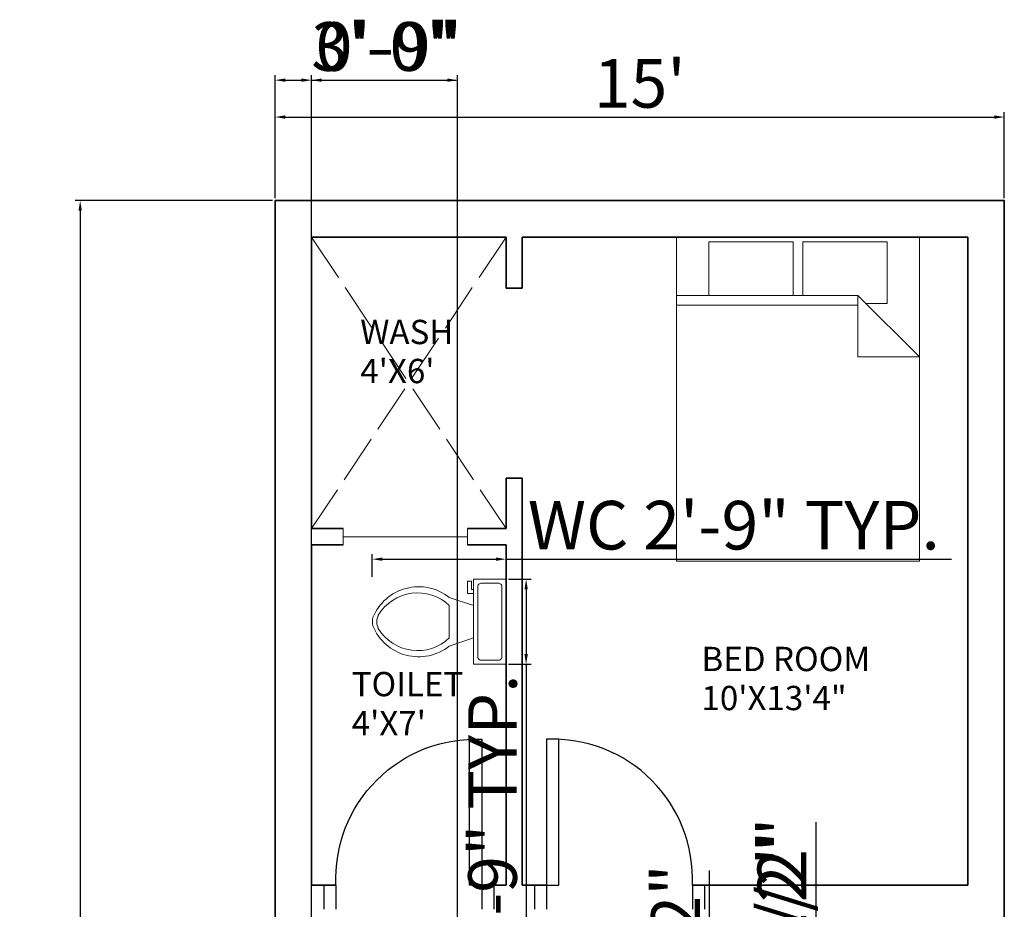
# Model space of a CAD drawing. Units: inches. Extents: x 2353 to 2961, y 642 to 1248.
# Tile 4 of 5: x 2353 to 2596, y 1025 to 1245. Entities that reach past the tile are written whole.
import ezdxf

# ---------------------------------------------------------------- set-up
doc = ezdxf.new("R2010")
doc.units = ezdxf.units.IN
doc.linetypes.add('ACAD_ISO02W100', pattern=[15, 12, -3])
for name, color, linetype, lineweight in [('A-ANNO-DIMS', 2, 'Continuous', 18), ('A-AREA-IDEN', 7, 'Continuous', 18), ('A-DOOR', 4, 'Continuous', 25), ('A-FLOR-FIXT', 9, 'Continuous', 18), ('A-FLOR-OPEN', 8, 'ACAD_ISO02W100', 13), ('A-FURN', 8, 'Continuous', 18), ('A-GLAZ', 4, 'Continuous', 18), ('A-WALL', 7, 'Continuous', 35)]:
    doc.layers.add(name, color=color, linetype=linetype, lineweight=lineweight)
doc.styles.get("Standard").update_dxf_attribs({"font": 'arial.ttf'})
doc.dimstyles.new('ISO-25', dxfattribs={"dimtxt": 12, "dimasz": 2.5, "dimexe": 1.25, "dimexo": 0.625, "dimtad": 1, "dimdec": 1, "dimlunit": 3, "dimtxsty": 'Standard', "dimcen": 2.5, "dimadec": 0, "dimazin": 0, "dimtfac": 1, "dimtdec": 1, "dimtmove": 0, "dimatfit": 3, "dimfxl": 1, "dimarcsym": 0})

# ---------------------------------------------------------------- blocks, each defined once
blk = doc.blocks.new('Bed - Queen')
for p, q in [((0, -80.00003), (0, 0)), ((0, 0), (59.99999, 0)), ((59.99999, 0), (59.99999, -80.00003)), ((7.99999, -1.2), (28.79998, -1.2)), ((7.99999, -14.4), (7.99999, -1.2)), ((28.79998, -1.2), (28.79998, -14.4)), ((31.19999, -1.2), (51.99999, -1.2)), ((31.19999, -14.4), (31.19999, -1.2)), ((51.99999, -1.2), (51.99999, -16.4)), ((0, -14.4), (44.8, -14.4)), ((59.99999, -29.6), (44.8, -14.4)), ((44.8, -14.4), (44.8, -29.6)), ((44.8, -16.8), (0, -16.8)), ((51.99999, -16.4), (46.79936, -16.4)), ((44.8, -29.6), (59.99999, -29.6)), ((59.99999, -80.00003), (0, -80.00003))]:
    blk.add_line(p, q)
blk = doc.blocks.new('Toilet - top')
for p, q in [((9.5, -6), (9.5, -2)), ((-10, -8.5), (-8, -8.5)), ((-10, -9.5), (-10, -8.5)), ((-7, -9.5), (-10, -9.5)), ((-8, -8.5), (-8, -8)), ((-7, -8), (-7, -9.5)), ((-4, -8), (-6, -14)), ((4, -8), (6, -14)), ((4, -14), (-4, -14))]:
    blk.add_line(p, q)
blk.add_lwpolyline([(10.5, -8), (10.5, 0), (-10.5, 0), (-10.5, -8)], close=True)
for points in [[(-9.5, -2), (-9.5, -6)], [(8.5, -1), (-8.5, -1)], [(-8.5, -7), (8.5, -7)]]:
    blk.add_lwpolyline(points)
for centre, radius, start, end in [((-8.62, -1.88), 0.884, 81.8699, 188.1301), ((8.62, -1.88), 0.884, 351.8699, 98.1301), ((-8.62, -6.12), 0.884, 171.8699, 278.1301), ((8.62, -6.12), 0.884, 261.8699, 8.1301), ((3.52, -21.58), 12.17, 141.4691, 247.9714), ((4.2, -21.82), 11.33, 136.3677, 238.9468), ((-3.52, -21.58), 12.17, 292.0284, 38.5307), ((-4.2, -21.82), 11.33, 301.053, 43.6321), ((0, -27.88), 4, 245.7318, 294.2682), ((0, -29), 4, 254.8605, 285.1395)]:
    blk.add_arc(centre, radius, start, end)
blk = doc.blocks.new('*D8')
at = {"layer": 'A-ANNO-DIMS', "color": 0, "lineweight": -2, "transparency": 16777216}
for p, q in [((2415.1, 1200.48), (2366.34, 1200.48)), ((2367.59, 1197.98), (2367.59, 722.98)), ((2415.1, 720.48), (2366.34, 720.48))]:
    blk.add_line(p, q, dxfattribs=at)
at = {"layer": 'A-ANNO-DIMS', "color": 0, "transparency": 16777216}
for points in [[(2367.17, 1197.98), (2368.01, 1197.98), (2367.59, 1200.48)], [(2367.17, 722.98), (2368.01, 722.98), (2367.59, 720.48)]]:
    blk.add_solid(points, dxfattribs=at)
at = {"layer": 'Defpoints', "color": 0, "transparency": 16777216}
for p in [(2415.72, 1200.48), (2367.59, 720.48), (2415.72, 720.48)]:
    blk.add_point(p, dxfattribs=at)
at = {"layer": 'A-ANNO-DIMS', "color": 0, "transparency": 16777216, "insert": (2360.84, 960.48), "char_height": 12, "attachment_point": 5, "rotation": 90}
blk.add_mtext("40'", dxfattribs=at)
blk = doc.blocks.new('*D12')
at = {"layer": 'A-ANNO-DIMS', "color": 0, "lineweight": -2, "transparency": 16777216}
for p, q in [((2415.72, 1201.11), (2415.72, 1222.37)), ((2418.22, 1221.12), (2593.22, 1221.12)), ((2595.72, 1201.11), (2595.72, 1222.37))]:
    blk.add_line(p, q, dxfattribs=at)
at = {"layer": 'A-ANNO-DIMS', "color": 0, "transparency": 16777216}
for points in [[(2418.22, 1221.54), (2418.22, 1220.71), (2415.72, 1221.12)], [(2593.22, 1221.54), (2593.22, 1220.71), (2595.72, 1221.12)]]:
    blk.add_solid(points, dxfattribs=at)
at = {"layer": 'Defpoints', "color": 0, "transparency": 16777216}
for p in [(2595.72, 1221.12), (2415.72, 1200.48), (2595.72, 1200.48)]:
    blk.add_point(p, dxfattribs=at)
at = {"layer": 'A-ANNO-DIMS', "color": 0, "transparency": 16777216, "insert": (2505.72, 1227.88), "char_height": 12, "attachment_point": 5}
blk.add_mtext("15'", dxfattribs=at)
blk = doc.blocks.new('DOOR-SINGLE-36IN')
for p, q in [((0, 6), (0, 0)), ((3, 6), (3, 0)), ((39, 6), (39, 0)), ((42, 6), (42, 0))]:
    blk.add_line(p, q)
blk.add_lwpolyline([(3, 6), (6, 6), (6, 42), (3, 42)], close=True)
blk.add_arc((4.5, 7.5), 34.53, 357.5104, 92.4896)
blk = doc.blocks.new('WASH-COURT-CROSS-4X6')
for p, q in [((0, 72), (48, 0)), ((48, 72), (0, 0))]:
    blk.add_line(p, q)
blk = doc.blocks.new('*D19')
at = {"layer": 'A-ANNO-DIMS', "color": 0, "lineweight": -2, "transparency": 16777216}
for p, q in [((2439.68, 1107.62), (2439.68, 1113.2)), ((2442.18, 1111.95), (2470.22, 1111.95)), ((2472.72, 1107.62), (2472.72, 1113.2)), ((2472.72, 1111.95), (2582.7, 1111.95))]:
    blk.add_line(p, q, dxfattribs=at)
at = {"layer": 'A-ANNO-DIMS', "color": 0, "transparency": 16777216}
for points in [[(2442.18, 1112.36), (2442.18, 1111.53), (2439.68, 1111.95)], [(2470.22, 1112.36), (2470.22, 1111.53), (2472.72, 1111.95)]]:
    blk.add_solid(points, dxfattribs=at)
at = {"layer": 'Defpoints', "color": 0, "transparency": 16777216}
for p in [(2472.72, 1111.95), (2439.68, 1106.99), (2472.72, 1106.99)]:
    blk.add_point(p, dxfattribs=at)
at = {"layer": 'A-ANNO-DIMS', "color": 0, "transparency": 16777216, "insert": (2528.96, 1118.78), "char_height": 12, "attachment_point": 5}
blk.add_mtext('WC 2\'-9" TYP.', dxfattribs=at)
blk = doc.blocks.new('*D20')
at = {"layer": 'A-ANNO-DIMS', "color": 0, "lineweight": -2, "transparency": 16777216}
for p, q in [((2473.35, 1106.99), (2478.93, 1106.99)), ((2477.68, 1104.49), (2477.68, 1088.49)), ((2473.35, 1085.99), (2478.93, 1085.99)), ((2477.68, 1085.99), (2477.68, 1010.22))]:
    blk.add_line(p, q, dxfattribs=at)
at = {"layer": 'A-ANNO-DIMS', "color": 0, "transparency": 16777216}
for points in [[(2477.26, 1104.49), (2478.1, 1104.49), (2477.68, 1106.99)], [(2477.26, 1088.49), (2478.1, 1088.49), (2477.68, 1085.99)]]:
    blk.add_solid(points, dxfattribs=at)
at = {"layer": 'Defpoints', "color": 0, "transparency": 16777216}
for p in [(2472.72, 1106.99), (2472.72, 1085.99), (2477.68, 1085.99)]:
    blk.add_point(p, dxfattribs=at)
at = {"layer": 'A-ANNO-DIMS', "color": 0, "transparency": 16777216, "insert": (2470.93, 1046.86), "char_height": 12, "attachment_point": 5, "rotation": 90}
blk.add_mtext('1\'-9" TYP.', dxfattribs=at)
blk = doc.blocks.new('*D22')
at = {"layer": 'A-ANNO-DIMS', "color": 0, "lineweight": -2, "transparency": 16777216}
for p, q in [((2522.95, 971.22), (2522.95, 1035.04)), ((2528.38, 971.22), (2521.7, 971.22)), ((2522.95, 949.04), (2522.95, 968.72)), ((2528.38, 946.54), (2521.7, 946.54))]:
    blk.add_line(p, q, dxfattribs=at)
at = {"layer": 'A-ANNO-DIMS', "color": 0, "transparency": 16777216}
for points in [[(2522.54, 968.72), (2523.37, 968.72), (2522.95, 971.22)], [(2522.54, 949.04), (2523.37, 949.04), (2522.95, 946.54)]]:
    blk.add_solid(points, dxfattribs=at)
at = {"layer": 'Defpoints', "color": 0, "transparency": 16777216}
for p in [(2522.95, 971.22), (2529.01, 971.22), (2529.01, 946.54)]:
    blk.add_point(p, dxfattribs=at)
at = {"layer": 'A-ANNO-DIMS', "color": 0, "transparency": 16777216, "insert": (2516.12, 1004.38), "char_height": 12, "attachment_point": 5, "rotation": 90}
blk.add_mtext('2\'-0 1/2"', dxfattribs=at)
blk = doc.blocks.new('*D35')
at = {"layer": 'A-ANNO-DIMS', "color": 0, "lineweight": -2, "transparency": 16777216}
for p, q in [((2424.72, 880.11), (2424.72, 1231.48)), ((2427.22, 1230.23), (2458.22, 1230.23)), ((2460.72, 880.11), (2460.72, 1231.48))]:
    blk.add_line(p, q, dxfattribs=at)
at = {"layer": 'A-ANNO-DIMS', "color": 0, "transparency": 16777216}
for points in [[(2427.22, 1230.65), (2427.22, 1229.82), (2424.72, 1230.23)], [(2458.22, 1230.65), (2458.22, 1229.82), (2460.72, 1230.23)]]:
    blk.add_solid(points, dxfattribs=at)
at = {"layer": 'Defpoints', "color": 0, "transparency": 16777216}
for p in [(2460.72, 1230.23), (2424.72, 879.48), (2460.72, 879.48)]:
    blk.add_point(p, dxfattribs=at)
at = {"layer": 'A-ANNO-DIMS', "color": 0, "transparency": 16777216, "insert": (2442.72, 1236.99), "char_height": 12, "attachment_point": 5}
blk.add_mtext('3\'-0"', dxfattribs=at)
blk = doc.blocks.new('*D38')
at = {"layer": 'A-ANNO-DIMS', "color": 0, "lineweight": -2, "transparency": 16777216}
for p, q in [((2415.72, 1201.11), (2415.72, 1231.48)), ((2418.22, 1230.23), (2422.22, 1230.23)), ((2424.72, 1192.11), (2424.72, 1231.48)), ((2424.72, 1230.23), (2460.37, 1230.23))]:
    blk.add_line(p, q, dxfattribs=at)
at = {"layer": 'A-ANNO-DIMS', "color": 0, "transparency": 16777216}
for points in [[(2418.22, 1230.65), (2418.22, 1229.82), (2415.72, 1230.23)], [(2422.22, 1230.65), (2422.22, 1229.82), (2424.72, 1230.23)]]:
    blk.add_solid(points, dxfattribs=at)
at = {"layer": 'Defpoints', "color": 0, "transparency": 16777216}
for p in [(2424.72, 1230.23), (2415.72, 1200.48), (2424.72, 1191.48)]:
    blk.add_point(p, dxfattribs=at)
at = {"layer": 'A-ANNO-DIMS', "color": 0, "transparency": 16777216, "insert": (2443.8, 1236.98), "char_height": 12, "attachment_point": 5}
blk.add_mtext('0\'-9"', dxfattribs=at)
blk = doc.blocks.new('*D48')
at = {"layer": 'A-ANNO-DIMS', "color": 0, "lineweight": -2, "transparency": 16777216}
for p, q in [((2549.2, 1047.02), (2549.2, 971.93)), ((2549.2, 928.87), (2549.2, 969.43))]:
    blk.add_line(p, q, dxfattribs=at)
at = {"layer": 'A-ANNO-DIMS', "color": 0, "transparency": 16777216}
blk.add_solid([(2548.78, 971.93), (2549.62, 971.93), (2549.2, 969.43)], dxfattribs=at)
at = {"layer": 'Defpoints', "color": 0, "transparency": 16777216}
for p in [(2549.2, 969.43), (2549.2, 928.87)]:
    blk.add_point(p, dxfattribs=at)
at = {"layer": 'A-ANNO-DIMS', "color": 0, "transparency": 16777216, "insert": (2542.37, 1010.72), "char_height": 12, "attachment_point": 5, "rotation": 90}
blk.add_mtext('R3\'-4 1/2"', dxfattribs=at)
blk = doc.blocks.new('*D49')
at = {"layer": 'A-ANNO-DIMS', "color": 0, "lineweight": -2, "transparency": 16777216}
for p, q in [((2549.2, 1042.98), (2549.2, 967.89)), ((2549.2, 928.11), (2549.2, 965.39))]:
    blk.add_line(p, q, dxfattribs=at)
at = {"layer": 'A-ANNO-DIMS', "color": 0, "transparency": 16777216}
blk.add_solid([(2548.78, 967.89), (2549.62, 967.89), (2549.2, 965.39)], dxfattribs=at)
at = {"layer": 'Defpoints', "color": 0, "transparency": 16777216}
for p in [(2549.2, 965.39), (2549.2, 928.11)]:
    blk.add_point(p, dxfattribs=at)
at = {"layer": 'A-ANNO-DIMS', "color": 0, "transparency": 16777216, "insert": (2542.37, 1006.68), "char_height": 12, "attachment_point": 5, "rotation": 90}
blk.add_mtext('R3\'-1 1/2"', dxfattribs=at)

msp = doc.modelspace()

# ---------------------------------------------------------------- linework, layer by layer
at = {"layer": 'A-GLAZ'}
for p, q in [((2432.49, 1119.48), (2432.49, 1115.48)), ((2463.2, 1119.48), (2463.2, 1115.48)), ((2432.49, 1117.48), (2463.2, 1117.48))]:
    msp.add_line(p, q, dxfattribs=at)
at = {"layer": 'A-WALL'}
for p, q in [((2424.72, 1191.48), (2424.72, 1119.48)), ((2472.72, 1191.48), (2424.72, 1191.48)), ((2472.72, 1191.48), (2472.72, 1178.85)), ((2586.72, 1191.48), (2476.72, 1191.48)), ((2476.72, 1191.48), (2476.72, 1178.85)), ((2586.72, 1031.48), (2586.72, 1191.48)), ((2472.72, 1178.85), (2476.72, 1178.85)), ((2472.72, 1131.91), (2476.72, 1131.91)), ((2472.72, 1131.91), (2472.72, 1119.48)), ((2476.72, 1131.91), (2476.72, 1031.48)), ((2432.49, 1119.48), (2424.72, 1119.48)), ((2472.72, 1119.48), (2463.2, 1119.48)), ((2424.72, 1115.48), (2424.72, 1031.48)), ((2432.49, 1115.48), (2424.72, 1115.48)), ((2472.72, 1115.48), (2463.2, 1115.48)), ((2472.72, 1115.48), (2472.72, 1031.48)), ((2430.72, 1031.48), (2424.72, 1031.48)), ((2472.72, 1031.48), (2466.72, 1031.48)), ((2482.72, 1031.48), (2476.72, 1031.48)), ((2586.72, 1031.48), (2518.72, 1031.48))]:
    msp.add_line(p, q, dxfattribs=at)
msp.add_lwpolyline([(2574.3, 720.48), (2595.72, 720.48), (2595.72, 1200.48), (2415.72, 1200.48), (2415.72, 720.48), (2445.67, 720.48)], dxfattribs=at)

# ---------------------------------------------------------------- block references
at = {"layer": 'A-DOOR', "extrusion": (0, 0, -1), "zscale": -1}
msp.add_blockref('DOOR-SINGLE-36IN', (-2469.72, 1025.48), dxfattribs=at)
at = {"layer": 'A-DOOR'}
msp.add_blockref('DOOR-SINGLE-36IN', (2479.72, 1025.48), dxfattribs=at)
at = {"layer": 'A-FLOR-FIXT', "rotation": 270}
msp.add_blockref('Toilet - top', (2472.72, 1096.49), dxfattribs=at)
at = {"layer": 'A-FLOR-OPEN'}
msp.add_blockref('WASH-COURT-CROSS-4X6', (2424.72, 1119.48), dxfattribs=at)
at = {"layer": 'A-FURN'}
msp.add_blockref('Bed - Queen', (2514.78, 1191.48), dxfattribs=at)

# ---------------------------------------------------------------- texts
at = {"layer": 'A-AREA-IDEN'}
for s, p in [('WASH', (2436.74, 1165.05)), ("4'X6'", (2436.74, 1155.41)), ('BED ROOM', (2520.96, 1084.3)), ('TOILET', (2434.62, 1078.1)), ('10\'X13\'4"', (2520.96, 1074.66)), ("4'X7'", (2434.62, 1068.46))]:
    msp.add_text(s, height=6, dxfattribs=at).set_placement(p)

# ---------------------------------------------------------------- dimensions: what is measured, and where the dimension line sits
at = {"layer": 'A-ANNO-DIMS'}
for base, p1, p2, override, picture, middle in [((2424.72, 1230.23), (2415.72, 1200.48), (2424.72, 1191.48), {"dimdec": 1, "dimlfac": 1, "dimrnd": 0, "dimzin": 1, "dimdsep": 46, "dimlunit": 4, "dimfrac": 2}, '*D38', (2443.8, 1236.98)), ((2460.72, 1230.23), (2424.72, 879.48), (2460.72, 879.48), {"dimdec": 1, "dimlfac": 1, "dimrnd": 0, "dimzin": 1, "dimdsep": 46, "dimlunit": 4, "dimfrac": 2}, '*D35', (2442.72, 1236.99)), ((2595.72, 1221.12), (2415.72, 1200.48), (2595.72, 1200.48), {"dimclrd": 0, "dimclre": 0, "dimclrt": 0}, '*D12', (2505.72, 1227.88))]:
    dim = msp.add_linear_dim(base=base, p1=p1, p2=p2, dimstyle='ISO-25', override=override, dxfattribs=at)
    dim.commit()
    dim.dimension.update_dxf_attribs({"geometry": picture, "text_midpoint": middle})
for base, p1, p2, override, picture, middle in [((2367.59, 720.48), (2415.72, 1200.48), (2415.72, 720.48), {"dimclrd": 0, "dimclre": 0, "dimclrt": 0}, '*D8', (2360.84, 960.48)), ((2522.95, 971.22), (2529.01, 946.54), (2529.01, 971.22), {"dimdec": 1, "dimlfac": 1, "dimrnd": 0, "dimzin": 1, "dimdsep": 46, "dimlunit": 4, "dimfrac": 2}, '*D22', (2516.12, 1004.38))]:
    dim = msp.add_linear_dim(base=base, p1=p1, p2=p2, angle=90, dimstyle='ISO-25', override=override, dxfattribs=at)
    dim.commit()
    dim.dimension.update_dxf_attribs({"geometry": picture, "text_midpoint": middle})
dim = msp.add_linear_dim(base=(2472.72, 1111.95), p1=(2439.68, 1106.99), p2=(2472.72, 1106.99), text='WC <> TYP.', dimstyle='ISO-25', override={"dimdec": 1, "dimlfac": 1, "dimrnd": 0, "dimzin": 1, "dimdsep": 46, "dimlunit": 4, "dimfrac": 2}, dxfattribs=at)
dim.commit()
dim.dimension.update_dxf_attribs({"geometry": '*D19', "text_midpoint": (2528.96, 1118.78)})
dim = msp.add_linear_dim(base=(2477.68, 1085.99), p1=(2472.72, 1106.99), p2=(2472.72, 1085.99), angle=270, text='<> TYP.', dimstyle='ISO-25', override={"dimdec": 1, "dimlfac": 1, "dimrnd": 0, "dimzin": 1, "dimdsep": 46, "dimlunit": 4, "dimfrac": 2}, dxfattribs=at)
dim.commit()
dim.dimension.update_dxf_attribs({"geometry": '*D20', "text_midpoint": (2470.93, 1046.86)})
for center, mpoint, picture, middle in [((2549.2, 928.87), (2549.2, 969.43), '*D48', (2542.37, 1010.72)), ((2549.2, 928.11), (2549.2, 965.39), '*D49', (2542.37, 1006.68))]:
    dim = msp.add_radius_dim(center=center, mpoint=mpoint, dimstyle='ISO-25', override={"dimdec": 1, "dimlfac": 1, "dimrnd": 0, "dimzin": 1, "dimdsep": 46, "dimlunit": 4, "dimfrac": 2}, dxfattribs=at)
    dim.commit()
    dim.dimension.update_dxf_attribs({"geometry": picture, "text_midpoint": middle})

doc.saveas('drawing.dxf')
